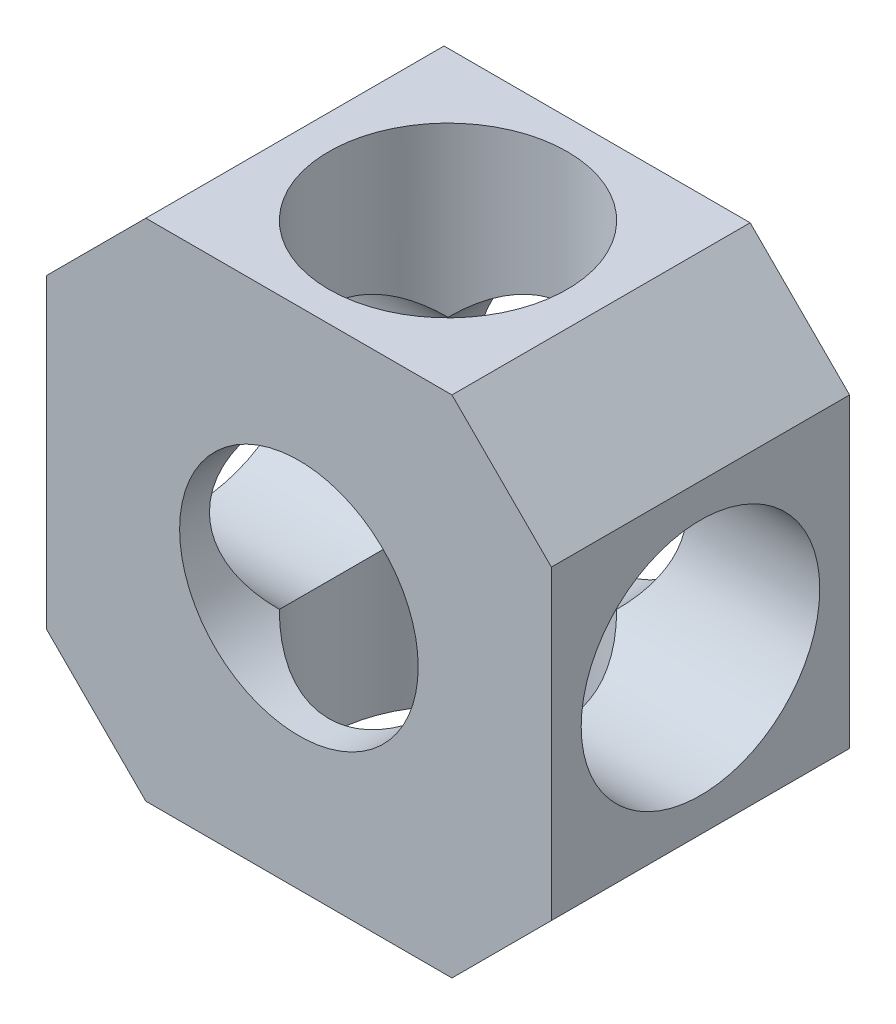
ISO-10303-21;
HEADER;
FILE_DESCRIPTION(('STEP AP214'),'2;1');
FILE_NAME('part.step','',(''),(''),'','','');
FILE_SCHEMA(('AUTOMOTIVE_DESIGN { 1 0 10303 214 1 1 1 1 }'));
ENDSEC;
DATA;
#1=APPLICATION_CONTEXT('core data for automotive mechanical design processes');
#2=APPLICATION_PROTOCOL_DEFINITION('international standard','automotive_design',2000,#1);
#3=PRODUCT_CONTEXT('',#1,'mechanical');
#4=PRODUCT('Part','Part','',(#3));
#5=PRODUCT_RELATED_PRODUCT_CATEGORY('part','',(#4));
#6=PRODUCT_DEFINITION_FORMATION('','',#4);
#7=PRODUCT_DEFINITION_CONTEXT('part definition',#1,'design');
#8=PRODUCT_DEFINITION('design','',#6,#7);
#9=PRODUCT_DEFINITION_SHAPE('','',#8);
#10=(LENGTH_UNIT() NAMED_UNIT(*) SI_UNIT(.MILLI.,.METRE.));
#11=(NAMED_UNIT(*) PLANE_ANGLE_UNIT() SI_UNIT($,.RADIAN.));
#12=(NAMED_UNIT(*) SI_UNIT($,.STERADIAN.) SOLID_ANGLE_UNIT());
#13=UNCERTAINTY_MEASURE_WITH_UNIT(LENGTH_MEASURE(1.E-05),#10,'distance_accuracy_value','');
#14=(GEOMETRIC_REPRESENTATION_CONTEXT(3) GLOBAL_UNCERTAINTY_ASSIGNED_CONTEXT((#13)) GLOBAL_UNIT_ASSIGNED_CONTEXT((#10,
#11,#12)) REPRESENTATION_CONTEXT('',''));
#15=CARTESIAN_POINT('',(0.,0.,0.));
#16=DIRECTION('',(0.,0.,1.));
#17=DIRECTION('',(1.,0.,0.));
#18=AXIS2_PLACEMENT_3D('',#15,#16,#17);
#19=CARTESIAN_POINT('',(0.,0.,7.5));
#20=DIRECTION('',(0.,0.,-1.));
#21=DIRECTION('',(-1.,0.,0.));
#22=AXIS2_PLACEMENT_3D('',#19,#20,#21);
#23=CYLINDRICAL_SURFACE('',#22,6.);
#24=CARTESIAN_POINT('',(0.,0.,-7.5));
#25=DIRECTION('',(0.,0.,-1.));
#26=DIRECTION('',(-1.,0.,0.));
#27=AXIS2_PLACEMENT_3D('',#24,#25,#26);
#28=CIRCLE('',#27,6.);
#29=CARTESIAN_POINT('',(-6.,0.,-7.5));
#30=VERTEX_POINT('',#29);
#31=EDGE_CURVE('E212',#30,#30,#28,.T.);
#32=ORIENTED_EDGE('',*,*,#31,.T.);
#33=EDGE_LOOP('',(#32));
#34=FACE_BOUND('',#33,.T.);
#35=CARTESIAN_POINT('',(0.,0.,0.));
#36=DIRECTION('',(0.707106781186547,0.,-0.707106781186547));
#37=DIRECTION('',(-0.707106781186547,0.,-0.707106781186547));
#38=AXIS2_PLACEMENT_3D('',#35,#36,#37);
#39=ELLIPSE('',#38,8.48528137423857,6.);
#40=CARTESIAN_POINT('',(-4.24264068711929,4.24264068711929,-4.24264068711929));
#41=VERTEX_POINT('',#40);
#42=CARTESIAN_POINT('',(-4.24264068711929,-4.24264068711929,-4.24264068711929));
#43=VERTEX_POINT('',#42);
#44=EDGE_CURVE('E137',#41,#43,#39,.F.);
#45=ORIENTED_EDGE('',*,*,#44,.T.);
#46=CARTESIAN_POINT('',(0.,0.,0.));
#47=DIRECTION('',(0.,0.707106781186547,-0.707106781186547));
#48=DIRECTION('',(0.,-0.707106781186547,-0.707106781186547));
#49=AXIS2_PLACEMENT_3D('',#46,#47,#48);
#50=ELLIPSE('',#49,8.48528137423857,6.);
#51=CARTESIAN_POINT('',(4.24264068711929,-4.24264068711929,-4.24264068711929));
#52=VERTEX_POINT('',#51);
#53=EDGE_CURVE('E128',#43,#52,#50,.F.);
#54=ORIENTED_EDGE('',*,*,#53,.T.);
#55=CARTESIAN_POINT('',(0.,0.,0.));
#56=DIRECTION('',(-0.707106781186547,0.,-0.707106781186547));
#57=DIRECTION('',(0.707106781186547,0.,-0.707106781186547));
#58=AXIS2_PLACEMENT_3D('',#55,#56,#57);
#59=ELLIPSE('',#58,8.48528137423857,6.);
#60=CARTESIAN_POINT('',(4.24264068711929,4.24264068711929,-4.24264068711929));
#61=VERTEX_POINT('',#60);
#62=EDGE_CURVE('E135',#52,#61,#59,.F.);
#63=ORIENTED_EDGE('',*,*,#62,.T.);
#64=CARTESIAN_POINT('',(0.,0.,0.));
#65=DIRECTION('',(0.,-0.707106781186547,-0.707106781186547));
#66=DIRECTION('',(0.,0.707106781186547,-0.707106781186547));
#67=AXIS2_PLACEMENT_3D('',#64,#65,#66);
#68=ELLIPSE('',#67,8.48528137423857,6.);
#69=EDGE_CURVE('E60',#61,#41,#68,.F.);
#70=ORIENTED_EDGE('',*,*,#69,.T.);
#71=EDGE_LOOP('',(#45,#54,#63,#70));
#72=FACE_BOUND('',#71,.T.);
#73=ADVANCED_FACE('F41',(#34,#72),#23,.F.);
#74=CARTESIAN_POINT('',(12.7,-12.7,7.5));
#75=DIRECTION('',(-1.,0.,0.));
#76=DIRECTION('',(0.,0.,1.));
#77=AXIS2_PLACEMENT_3D('',#74,#75,#76);
#78=PLANE('',#77);
#79=CARTESIAN_POINT('',(12.7,0.,0.));
#80=DIRECTION('',(-1.,0.,0.));
#81=DIRECTION('',(0.,0.,1.));
#82=AXIS2_PLACEMENT_3D('',#79,#80,#81);
#83=CIRCLE('',#82,6.);
#84=CARTESIAN_POINT('',(12.7,0.,6.));
#85=VERTEX_POINT('',#84);
#86=EDGE_CURVE('E216',#85,#85,#83,.T.);
#87=ORIENTED_EDGE('',*,*,#86,.T.);
#88=EDGE_LOOP('',(#87));
#89=FACE_BOUND('',#88,.T.);
#90=DIRECTION('',(0.,1.,0.));
#91=VECTOR('',#90,1.);
#92=CARTESIAN_POINT('',(12.7,-12.7,-7.5));
#93=LINE('',#92,#91);
#94=CARTESIAN_POINT('',(12.7,-7.69999999999999,-7.5));
#95=VERTEX_POINT('',#94);
#96=CARTESIAN_POINT('',(12.7,7.69999999999999,-7.5));
#97=VERTEX_POINT('',#96);
#98=EDGE_CURVE('E198',#95,#97,#93,.T.);
#99=ORIENTED_EDGE('',*,*,#98,.T.);
#100=DIRECTION('',(0.,0.,1.));
#101=VECTOR('',#100,1.);
#102=CARTESIAN_POINT('',(12.7,7.69999999999999,7.5));
#103=LINE('',#102,#101);
#104=CARTESIAN_POINT('',(12.7,7.69999999999999,7.5));
#105=VERTEX_POINT('',#104);
#106=EDGE_CURVE('E167',#97,#105,#103,.T.);
#107=ORIENTED_EDGE('',*,*,#106,.T.);
#108=DIRECTION('',(0.,1.,0.));
#109=VECTOR('',#108,1.);
#110=CARTESIAN_POINT('',(12.7,-12.7,7.5));
#111=LINE('',#110,#109);
#112=CARTESIAN_POINT('',(12.7,-7.69999999999999,7.5));
#113=VERTEX_POINT('',#112);
#114=EDGE_CURVE('E195',#113,#105,#111,.T.);
#115=ORIENTED_EDGE('',*,*,#114,.F.);
#116=DIRECTION('',(0.,0.,-1.));
#117=VECTOR('',#116,1.);
#118=CARTESIAN_POINT('',(12.7,-7.69999999999999,7.5));
#119=LINE('',#118,#117);
#120=EDGE_CURVE('E175',#113,#95,#119,.T.);
#121=ORIENTED_EDGE('',*,*,#120,.T.);
#122=EDGE_LOOP('',(#99,#107,#115,#121));
#123=FACE_BOUND('',#122,.T.);
#124=ADVANCED_FACE('F253',(#89,#123),#78,.F.);
#125=CARTESIAN_POINT('',(-12.7,12.7,7.5));
#126=DIRECTION('',(0.,-1.,0.));
#127=DIRECTION('',(0.,0.,-1.));
#128=AXIS2_PLACEMENT_3D('',#125,#126,#127);
#129=PLANE('',#128);
#130=CARTESIAN_POINT('',(0.,12.7,0.));
#131=DIRECTION('',(0.,1.,0.));
#132=DIRECTION('',(0.,0.,1.));
#133=AXIS2_PLACEMENT_3D('',#130,#131,#132);
#134=CIRCLE('',#133,6.);
#135=CARTESIAN_POINT('',(0.,12.7,6.));
#136=VERTEX_POINT('',#135);
#137=EDGE_CURVE('E234',#136,#136,#134,.T.);
#138=ORIENTED_EDGE('',*,*,#137,.F.);
#139=EDGE_LOOP('',(#138));
#140=FACE_BOUND('',#139,.T.);
#141=DIRECTION('',(-1.,0.,0.));
#142=VECTOR('',#141,1.);
#143=CARTESIAN_POINT('',(-12.7,12.7,7.5));
#144=LINE('',#143,#142);
#145=CARTESIAN_POINT('',(7.69999999999999,12.7,7.5));
#146=VERTEX_POINT('',#145);
#147=CARTESIAN_POINT('',(-7.69999999999997,12.7,7.5));
#148=VERTEX_POINT('',#147);
#149=EDGE_CURVE('E206',#146,#148,#144,.T.);
#150=ORIENTED_EDGE('',*,*,#149,.F.);
#151=DIRECTION('',(0.,0.,-1.));
#152=VECTOR('',#151,1.);
#153=CARTESIAN_POINT('',(7.69999999999999,12.7,7.5));
#154=LINE('',#153,#152);
#155=CARTESIAN_POINT('',(7.69999999999999,12.7,-7.5));
#156=VERTEX_POINT('',#155);
#157=EDGE_CURVE('E182',#146,#156,#154,.T.);
#158=ORIENTED_EDGE('',*,*,#157,.T.);
#159=DIRECTION('',(-1.,0.,0.));
#160=VECTOR('',#159,1.);
#161=CARTESIAN_POINT('',(-12.7,12.7,-7.5));
#162=LINE('',#161,#160);
#163=CARTESIAN_POINT('',(-7.69999999999997,12.7,-7.5));
#164=VERTEX_POINT('',#163);
#165=EDGE_CURVE('E196',#156,#164,#162,.T.);
#166=ORIENTED_EDGE('',*,*,#165,.T.);
#167=DIRECTION('',(0.,0.,1.));
#168=VECTOR('',#167,1.);
#169=CARTESIAN_POINT('',(-7.69999999999997,12.7,7.5));
#170=LINE('',#169,#168);
#171=EDGE_CURVE('E187',#164,#148,#170,.T.);
#172=ORIENTED_EDGE('',*,*,#171,.T.);
#173=EDGE_LOOP('',(#150,#158,#166,#172));
#174=FACE_BOUND('',#173,.T.);
#175=ADVANCED_FACE('F263',(#140,#174),#129,.F.);
#176=CARTESIAN_POINT('',(-12.7,-12.7,7.5));
#177=DIRECTION('',(1.,0.,0.));
#178=DIRECTION('',(0.,0.,-1.));
#179=AXIS2_PLACEMENT_3D('',#176,#177,#178);
#180=PLANE('',#179);
#181=CARTESIAN_POINT('',(-12.7,0.,0.));
#182=DIRECTION('',(-1.,0.,0.));
#183=DIRECTION('',(0.,0.,1.));
#184=AXIS2_PLACEMENT_3D('',#181,#182,#183);
#185=CIRCLE('',#184,6.);
#186=CARTESIAN_POINT('',(-12.7,0.,6.));
#187=VERTEX_POINT('',#186);
#188=EDGE_CURVE('E218',#187,#187,#185,.T.);
#189=ORIENTED_EDGE('',*,*,#188,.F.);
#190=EDGE_LOOP('',(#189));
#191=FACE_BOUND('',#190,.T.);
#192=DIRECTION('',(0.,-1.,0.));
#193=VECTOR('',#192,1.);
#194=CARTESIAN_POINT('',(-12.7,-12.7,7.5));
#195=LINE('',#194,#193);
#196=CARTESIAN_POINT('',(-12.7,7.69999999999998,7.5));
#197=VERTEX_POINT('',#196);
#198=CARTESIAN_POINT('',(-12.7,-7.69999999999998,7.5));
#199=VERTEX_POINT('',#198);
#200=EDGE_CURVE('E202',#197,#199,#195,.T.);
#201=ORIENTED_EDGE('',*,*,#200,.F.);
#202=DIRECTION('',(0.,0.,-1.));
#203=VECTOR('',#202,1.);
#204=CARTESIAN_POINT('',(-12.7,7.69999999999998,7.5));
#205=LINE('',#204,#203);
#206=CARTESIAN_POINT('',(-12.7,7.69999999999998,-7.5));
#207=VERTEX_POINT('',#206);
#208=EDGE_CURVE('E160',#197,#207,#205,.T.);
#209=ORIENTED_EDGE('',*,*,#208,.T.);
#210=DIRECTION('',(0.,-1.,0.));
#211=VECTOR('',#210,1.);
#212=CARTESIAN_POINT('',(-12.7,-12.7,-7.5));
#213=LINE('',#212,#211);
#214=CARTESIAN_POINT('',(-12.7,-7.69999999999998,-7.5));
#215=VERTEX_POINT('',#214);
#216=EDGE_CURVE('E192',#207,#215,#213,.T.);
#217=ORIENTED_EDGE('',*,*,#216,.T.);
#218=DIRECTION('',(0.,0.,1.));
#219=VECTOR('',#218,1.);
#220=CARTESIAN_POINT('',(-12.7,-7.69999999999998,7.5));
#221=LINE('',#220,#219);
#222=EDGE_CURVE('E157',#215,#199,#221,.T.);
#223=ORIENTED_EDGE('',*,*,#222,.T.);
#224=EDGE_LOOP('',(#201,#209,#217,#223));
#225=FACE_BOUND('',#224,.T.);
#226=ADVANCED_FACE('F308',(#191,#225),#180,.F.);
#227=CARTESIAN_POINT('',(-12.7,-12.7,7.5));
#228=DIRECTION('',(0.,1.,0.));
#229=DIRECTION('',(0.,0.,1.));
#230=AXIS2_PLACEMENT_3D('',#227,#228,#229);
#231=PLANE('',#230);
#232=CARTESIAN_POINT('',(0.,-12.7,0.));
#233=DIRECTION('',(0.,1.,0.));
#234=DIRECTION('',(0.,0.,1.));
#235=AXIS2_PLACEMENT_3D('',#232,#233,#234);
#236=CIRCLE('',#235,6.);
#237=CARTESIAN_POINT('',(0.,-12.7,6.));
#238=VERTEX_POINT('',#237);
#239=EDGE_CURVE('E231',#238,#238,#236,.T.);
#240=ORIENTED_EDGE('',*,*,#239,.T.);
#241=EDGE_LOOP('',(#240));
#242=FACE_BOUND('',#241,.T.);
#243=DIRECTION('',(1.,0.,0.));
#244=VECTOR('',#243,1.);
#245=CARTESIAN_POINT('',(-12.7,-12.7,7.5));
#246=LINE('',#245,#244);
#247=CARTESIAN_POINT('',(-7.69999999999997,-12.7,7.5));
#248=VERTEX_POINT('',#247);
#249=CARTESIAN_POINT('',(7.69999999999999,-12.7,7.5));
#250=VERTEX_POINT('',#249);
#251=EDGE_CURVE('E189',#248,#250,#246,.T.);
#252=ORIENTED_EDGE('',*,*,#251,.F.);
#253=DIRECTION('',(0.,0.,-1.));
#254=VECTOR('',#253,1.);
#255=CARTESIAN_POINT('',(-7.69999999999997,-12.7,7.5));
#256=LINE('',#255,#254);
#257=CARTESIAN_POINT('',(-7.69999999999997,-12.7,-7.5));
#258=VERTEX_POINT('',#257);
#259=EDGE_CURVE('E152',#248,#258,#256,.T.);
#260=ORIENTED_EDGE('',*,*,#259,.T.);
#261=DIRECTION('',(1.,0.,0.));
#262=VECTOR('',#261,1.);
#263=CARTESIAN_POINT('',(-12.7,-12.7,-7.5));
#264=LINE('',#263,#262);
#265=CARTESIAN_POINT('',(7.69999999999999,-12.7,-7.5));
#266=VERTEX_POINT('',#265);
#267=EDGE_CURVE('E186',#258,#266,#264,.T.);
#268=ORIENTED_EDGE('',*,*,#267,.T.);
#269=DIRECTION('',(0.,0.,1.));
#270=VECTOR('',#269,1.);
#271=CARTESIAN_POINT('',(7.69999999999999,-12.7,7.5));
#272=LINE('',#271,#270);
#273=EDGE_CURVE('E155',#266,#250,#272,.T.);
#274=ORIENTED_EDGE('',*,*,#273,.T.);
#275=EDGE_LOOP('',(#252,#260,#268,#274));
#276=FACE_BOUND('',#275,.T.);
#277=ADVANCED_FACE('F239',(#242,#276),#231,.F.);
#278=CARTESIAN_POINT('',(0.,0.,7.5));
#279=DIRECTION('',(0.,0.,-1.));
#280=DIRECTION('',(-1.,0.,0.));
#281=AXIS2_PLACEMENT_3D('',#278,#279,#280);
#282=PLANE('',#281);
#283=CARTESIAN_POINT('',(0.,0.,7.5));
#284=DIRECTION('',(0.,0.,-1.));
#285=DIRECTION('',(-1.,0.,0.));
#286=AXIS2_PLACEMENT_3D('',#283,#284,#285);
#287=CIRCLE('',#286,6.);
#288=CARTESIAN_POINT('',(-6.,0.,7.5));
#289=VERTEX_POINT('',#288);
#290=EDGE_CURVE('E205',#289,#289,#287,.T.);
#291=ORIENTED_EDGE('',*,*,#290,.T.);
#292=EDGE_LOOP('',(#291));
#293=FACE_BOUND('',#292,.T.);
#294=ORIENTED_EDGE('',*,*,#114,.T.);
#295=DIRECTION('',(0.707106781186548,-0.707106781186548,0.));
#296=VECTOR('',#295,1.);
#297=CARTESIAN_POINT('',(7.69999999999999,12.7,7.5));
#298=LINE('',#297,#296);
#299=EDGE_CURVE('E162',#105,#146,#298,.F.);
#300=ORIENTED_EDGE('',*,*,#299,.T.);
#301=ORIENTED_EDGE('',*,*,#149,.T.);
#302=DIRECTION('',(0.707106781186548,0.707106781186548,0.));
#303=VECTOR('',#302,1.);
#304=CARTESIAN_POINT('',(-12.7,7.69999999999998,7.5));
#305=LINE('',#304,#303);
#306=EDGE_CURVE('E165',#148,#197,#305,.F.);
#307=ORIENTED_EDGE('',*,*,#306,.T.);
#308=ORIENTED_EDGE('',*,*,#200,.T.);
#309=DIRECTION('',(-0.707106781186548,0.707106781186548,0.));
#310=VECTOR('',#309,1.);
#311=CARTESIAN_POINT('',(-7.69999999999997,-12.7,7.5));
#312=LINE('',#311,#310);
#313=EDGE_CURVE('E168',#199,#248,#312,.F.);
#314=ORIENTED_EDGE('',*,*,#313,.T.);
#315=ORIENTED_EDGE('',*,*,#251,.T.);
#316=DIRECTION('',(-0.707106781186548,-0.707106781186548,0.));
#317=VECTOR('',#316,1.);
#318=CARTESIAN_POINT('',(12.7,-7.69999999999999,7.5));
#319=LINE('',#318,#317);
#320=EDGE_CURVE('E166',#250,#113,#319,.F.);
#321=ORIENTED_EDGE('',*,*,#320,.T.);
#322=EDGE_LOOP('',(#294,#300,#301,#307,#308,#314,#315,#321));
#323=FACE_BOUND('',#322,.T.);
#324=ADVANCED_FACE('F282',(#293,#323),#282,.F.);
#325=CARTESIAN_POINT('',(0.,0.,-7.5));
#326=DIRECTION('',(0.,0.,-1.));
#327=DIRECTION('',(-1.,0.,0.));
#328=AXIS2_PLACEMENT_3D('',#325,#326,#327);
#329=PLANE('',#328);
#330=ORIENTED_EDGE('',*,*,#31,.F.);
#331=EDGE_LOOP('',(#330));
#332=FACE_BOUND('',#331,.T.);
#333=ORIENTED_EDGE('',*,*,#165,.F.);
#334=DIRECTION('',(-0.707106781186548,0.707106781186548,0.));
#335=VECTOR('',#334,1.);
#336=CARTESIAN_POINT('',(10.2,10.2,-7.5));
#337=LINE('',#336,#335);
#338=EDGE_CURVE('E174',#156,#97,#337,.F.);
#339=ORIENTED_EDGE('',*,*,#338,.T.);
#340=ORIENTED_EDGE('',*,*,#98,.F.);
#341=DIRECTION('',(0.707106781186548,0.707106781186548,0.));
#342=VECTOR('',#341,1.);
#343=CARTESIAN_POINT('',(10.2,-10.2,-7.5));
#344=LINE('',#343,#342);
#345=EDGE_CURVE('E181',#95,#266,#344,.F.);
#346=ORIENTED_EDGE('',*,*,#345,.T.);
#347=ORIENTED_EDGE('',*,*,#267,.F.);
#348=DIRECTION('',(0.707106781186548,-0.707106781186548,0.));
#349=VECTOR('',#348,1.);
#350=CARTESIAN_POINT('',(-10.2,-10.2,-7.5));
#351=LINE('',#350,#349);
#352=EDGE_CURVE('E177',#258,#215,#351,.F.);
#353=ORIENTED_EDGE('',*,*,#352,.T.);
#354=ORIENTED_EDGE('',*,*,#216,.F.);
#355=DIRECTION('',(-0.707106781186548,-0.707106781186548,0.));
#356=VECTOR('',#355,1.);
#357=CARTESIAN_POINT('',(-10.2,10.2,-7.5));
#358=LINE('',#357,#356);
#359=EDGE_CURVE('E180',#207,#164,#358,.F.);
#360=ORIENTED_EDGE('',*,*,#359,.T.);
#361=EDGE_LOOP('',(#333,#339,#340,#346,#347,#353,#354,#360));
#362=FACE_BOUND('',#361,.T.);
#363=ADVANCED_FACE('F285',(#332,#362),#329,.T.);
#364=CARTESIAN_POINT('',(7.69999999999999,12.7,7.5));
#365=DIRECTION('',(-0.707106781186548,-0.707106781186548,0.));
#366=DIRECTION('',(0.,0.,-1.));
#367=AXIS2_PLACEMENT_3D('',#364,#365,#366);
#368=PLANE('',#367);
#369=ORIENTED_EDGE('',*,*,#299,.F.);
#370=ORIENTED_EDGE('',*,*,#106,.F.);
#371=ORIENTED_EDGE('',*,*,#338,.F.);
#372=ORIENTED_EDGE('',*,*,#157,.F.);
#373=EDGE_LOOP('',(#369,#370,#371,#372));
#374=FACE_BOUND('',#373,.T.);
#375=ADVANCED_FACE('F294',(#374),#368,.F.);
#376=CARTESIAN_POINT('',(-12.7,7.69999999999998,7.5));
#377=DIRECTION('',(0.707106781186547,-0.707106781186547,0.));
#378=DIRECTION('',(0.,0.,-1.));
#379=AXIS2_PLACEMENT_3D('',#376,#377,#378);
#380=PLANE('',#379);
#381=ORIENTED_EDGE('',*,*,#306,.F.);
#382=ORIENTED_EDGE('',*,*,#171,.F.);
#383=ORIENTED_EDGE('',*,*,#359,.F.);
#384=ORIENTED_EDGE('',*,*,#208,.F.);
#385=EDGE_LOOP('',(#381,#382,#383,#384));
#386=FACE_BOUND('',#385,.T.);
#387=ADVANCED_FACE('F304',(#386),#380,.F.);
#388=CARTESIAN_POINT('',(-7.69999999999997,-12.7,7.5));
#389=DIRECTION('',(0.707106781186547,0.707106781186547,0.));
#390=DIRECTION('',(0.,0.,-1.));
#391=AXIS2_PLACEMENT_3D('',#388,#389,#390);
#392=PLANE('',#391);
#393=ORIENTED_EDGE('',*,*,#313,.F.);
#394=ORIENTED_EDGE('',*,*,#222,.F.);
#395=ORIENTED_EDGE('',*,*,#352,.F.);
#396=ORIENTED_EDGE('',*,*,#259,.F.);
#397=EDGE_LOOP('',(#393,#394,#395,#396));
#398=FACE_BOUND('',#397,.T.);
#399=ADVANCED_FACE('F276',(#398),#392,.F.);
#400=CARTESIAN_POINT('',(12.7,-7.69999999999999,7.5));
#401=DIRECTION('',(-0.707106781186548,0.707106781186548,0.));
#402=DIRECTION('',(0.,0.,-1.));
#403=AXIS2_PLACEMENT_3D('',#400,#401,#402);
#404=PLANE('',#403);
#405=ORIENTED_EDGE('',*,*,#320,.F.);
#406=ORIENTED_EDGE('',*,*,#273,.F.);
#407=ORIENTED_EDGE('',*,*,#345,.F.);
#408=ORIENTED_EDGE('',*,*,#120,.F.);
#409=EDGE_LOOP('',(#405,#406,#407,#408));
#410=FACE_BOUND('',#409,.T.);
#411=ADVANCED_FACE('F42',(#410),#404,.F.);
#412=CARTESIAN_POINT('',(0.,0.,0.));
#413=DIRECTION('',(-0.707106781186547,0.,-0.707106781186547));
#414=DIRECTION('',(0.707106781186547,0.,-0.707106781186547));
#415=AXIS2_PLACEMENT_3D('',#412,#413,#414);
#416=ELLIPSE('',#415,8.48528137423857,6.);
#417=CARTESIAN_POINT('',(-4.24264068711929,-4.24264068711929,4.24264068711929));
#418=VERTEX_POINT('',#417);
#419=CARTESIAN_POINT('',(-4.24264068711929,4.24264068711929,4.24264068711929));
#420=VERTEX_POINT('',#419);
#421=EDGE_CURVE('E144',#418,#420,#416,.T.);
#422=ORIENTED_EDGE('',*,*,#421,.T.);
#423=CARTESIAN_POINT('',(0.,0.,0.));
#424=DIRECTION('',(0.,0.707106781186547,-0.707106781186547));
#425=DIRECTION('',(0.,-0.707106781186547,-0.707106781186547));
#426=AXIS2_PLACEMENT_3D('',#423,#424,#425);
#427=ELLIPSE('',#426,8.48528137423857,6.);
#428=CARTESIAN_POINT('',(4.24264068711929,4.24264068711929,4.24264068711929));
#429=VERTEX_POINT('',#428);
#430=EDGE_CURVE('E226',#420,#429,#427,.T.);
#431=ORIENTED_EDGE('',*,*,#430,.T.);
#432=CARTESIAN_POINT('',(0.,0.,0.));
#433=DIRECTION('',(0.707106781186547,0.,-0.707106781186547));
#434=DIRECTION('',(-0.707106781186547,0.,-0.707106781186547));
#435=AXIS2_PLACEMENT_3D('',#432,#433,#434);
#436=ELLIPSE('',#435,8.48528137423857,6.);
#437=CARTESIAN_POINT('',(4.24264068711929,-4.24264068711929,4.24264068711929));
#438=VERTEX_POINT('',#437);
#439=EDGE_CURVE('E150',#429,#438,#436,.T.);
#440=ORIENTED_EDGE('',*,*,#439,.T.);
#441=CARTESIAN_POINT('',(0.,0.,0.));
#442=DIRECTION('',(0.,-0.707106781186547,-0.707106781186547));
#443=DIRECTION('',(0.,0.707106781186547,-0.707106781186547));
#444=AXIS2_PLACEMENT_3D('',#441,#442,#443);
#445=ELLIPSE('',#444,8.48528137423857,6.);
#446=EDGE_CURVE('E63',#438,#418,#445,.T.);
#447=ORIENTED_EDGE('',*,*,#446,.T.);
#448=EDGE_LOOP('',(#422,#431,#440,#447));
#449=FACE_BOUND('',#448,.T.);
#450=ORIENTED_EDGE('',*,*,#290,.F.);
#451=EDGE_LOOP('',(#450));
#452=FACE_BOUND('',#451,.T.);
#453=ADVANCED_FACE('F257',(#449,#452),#23,.F.);
#454=CARTESIAN_POINT('',(12.7,0.,0.));
#455=DIRECTION('',(-1.,0.,0.));
#456=DIRECTION('',(0.,0.,1.));
#457=AXIS2_PLACEMENT_3D('',#454,#455,#456);
#458=CYLINDRICAL_SURFACE('',#457,6.);
#459=ORIENTED_EDGE('',*,*,#188,.T.);
#460=EDGE_LOOP('',(#459));
#461=FACE_BOUND('',#460,.T.);
#462=ORIENTED_EDGE('',*,*,#421,.F.);
#463=CARTESIAN_POINT('',(0.,0.,0.));
#464=DIRECTION('',(-0.707106781186547,0.707106781186547,0.));
#465=DIRECTION('',(-0.707106781186547,-0.707106781186547,0.));
#466=AXIS2_PLACEMENT_3D('',#463,#464,#465);
#467=ELLIPSE('',#466,8.48528137423857,6.);
#468=EDGE_CURVE('E142',#418,#43,#467,.F.);
#469=ORIENTED_EDGE('',*,*,#468,.T.);
#470=ORIENTED_EDGE('',*,*,#44,.F.);
#471=CARTESIAN_POINT('',(0.,0.,0.));
#472=DIRECTION('',(-0.707106781186547,-0.707106781186547,0.));
#473=DIRECTION('',(-0.707106781186547,0.707106781186547,0.));
#474=AXIS2_PLACEMENT_3D('',#471,#472,#473);
#475=ELLIPSE('',#474,8.48528137423857,6.);
#476=EDGE_CURVE('E225',#41,#420,#475,.F.);
#477=ORIENTED_EDGE('',*,*,#476,.T.);
#478=EDGE_LOOP('',(#462,#469,#470,#477));
#479=FACE_BOUND('',#478,.T.);
#480=ADVANCED_FACE('F252',(#461,#479),#458,.F.);
#481=ORIENTED_EDGE('',*,*,#86,.F.);
#482=EDGE_LOOP('',(#481));
#483=FACE_BOUND('',#482,.T.);
#484=ORIENTED_EDGE('',*,*,#439,.F.);
#485=CARTESIAN_POINT('',(0.,0.,0.));
#486=DIRECTION('',(-0.707106781186547,0.707106781186547,0.));
#487=DIRECTION('',(-0.707106781186547,-0.707106781186547,0.));
#488=AXIS2_PLACEMENT_3D('',#485,#486,#487);
#489=ELLIPSE('',#488,8.48528137423857,6.);
#490=EDGE_CURVE('E11',#429,#61,#489,.T.);
#491=ORIENTED_EDGE('',*,*,#490,.T.);
#492=ORIENTED_EDGE('',*,*,#62,.F.);
#493=CARTESIAN_POINT('',(0.,0.,0.));
#494=DIRECTION('',(-0.707106781186547,-0.707106781186547,0.));
#495=DIRECTION('',(-0.707106781186547,0.707106781186547,0.));
#496=AXIS2_PLACEMENT_3D('',#493,#494,#495);
#497=ELLIPSE('',#496,8.48528137423857,6.);
#498=EDGE_CURVE('E49',#52,#438,#497,.T.);
#499=ORIENTED_EDGE('',*,*,#498,.T.);
#500=EDGE_LOOP('',(#484,#491,#492,#499));
#501=FACE_BOUND('',#500,.T.);
#502=ADVANCED_FACE('F141',(#483,#501),#458,.F.);
#503=CARTESIAN_POINT('',(0.,-12.7,0.));
#504=DIRECTION('',(0.,1.,0.));
#505=DIRECTION('',(0.,0.,1.));
#506=AXIS2_PLACEMENT_3D('',#503,#504,#505);
#507=CYLINDRICAL_SURFACE('',#506,6.);
#508=ORIENTED_EDGE('',*,*,#239,.F.);
#509=EDGE_LOOP('',(#508));
#510=FACE_BOUND('',#509,.T.);
#511=ORIENTED_EDGE('',*,*,#446,.F.);
#512=ORIENTED_EDGE('',*,*,#498,.F.);
#513=ORIENTED_EDGE('',*,*,#53,.F.);
#514=ORIENTED_EDGE('',*,*,#468,.F.);
#515=EDGE_LOOP('',(#511,#512,#513,#514));
#516=FACE_BOUND('',#515,.T.);
#517=ADVANCED_FACE('F127',(#510,#516),#507,.F.);
#518=ORIENTED_EDGE('',*,*,#137,.T.);
#519=EDGE_LOOP('',(#518));
#520=FACE_BOUND('',#519,.T.);
#521=ORIENTED_EDGE('',*,*,#69,.F.);
#522=ORIENTED_EDGE('',*,*,#490,.F.);
#523=ORIENTED_EDGE('',*,*,#430,.F.);
#524=ORIENTED_EDGE('',*,*,#476,.F.);
#525=EDGE_LOOP('',(#521,#522,#523,#524));
#526=FACE_BOUND('',#525,.T.);
#527=ADVANCED_FACE('F242',(#520,#526),#507,.F.);
#528=CLOSED_SHELL('',(#73,#124,#175,#226,#277,#324,#363,#375,#387,#399,#411,#453,#480,#502,#517,#527));
#529=MANIFOLD_SOLID_BREP('B2',#528);
#530=ADVANCED_BREP_SHAPE_REPRESENTATION('',(#18,#529),#14);
#531=SHAPE_DEFINITION_REPRESENTATION(#9,#530);
ENDSEC;
END-ISO-10303-21;
